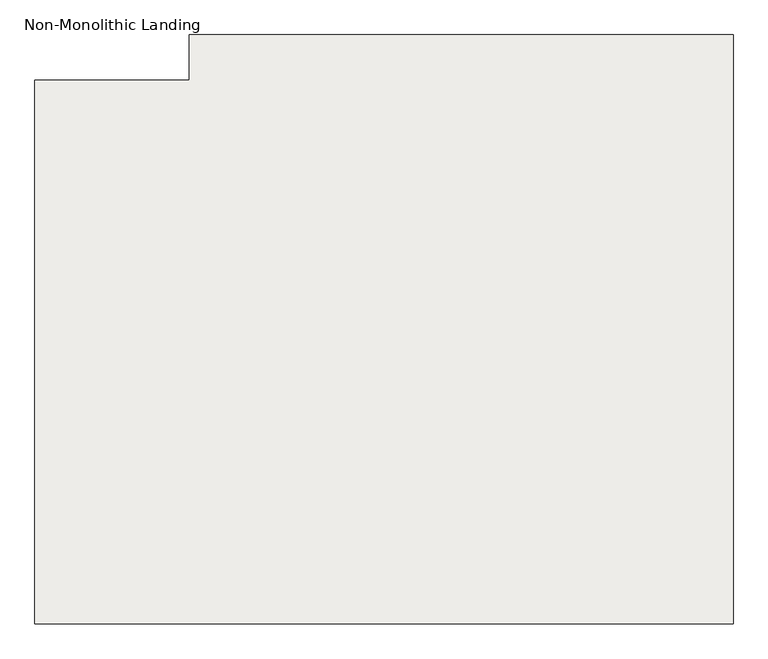
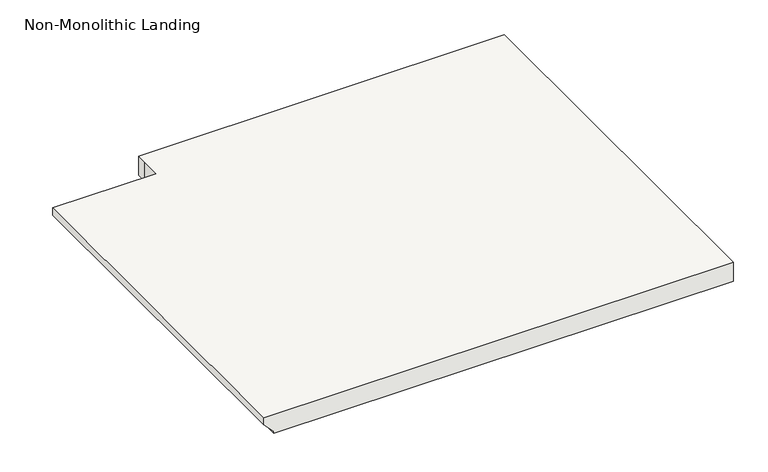
"""IFC4 building model written with IfcOpenShell, lengths in millimetres: slab geometry, Non-Monolithic Landing."""

from ifc_helpers import new_model, si_unit, origin, place, context, project, spatial, faceted_brep, source, transform, mapped, element, save


def non_monolithic_landing_c5e4f846(model_context):
    return source(origin(), model_context, "Body", "Brep", [
        faceted_brep([(9992.8923267, 6928.6147181, 2209.8), (9992.8923267, 7893.8147181, 2209.8), (9992.8923267, 7919.2147181, 2209.8), (9078.4923267, 7919.2147181, 2209.8), (9078.4923267, 7893.8147181, 2209.8), (9078.4923267, 7843.0147181, 2209.8), (8819.4175025, 7843.0147181, 2209.8), (8819.4175025, 6928.6147181, 2209.8), (8844.8175025, 6928.6147181, 2159.0), (8844.8175025, 7843.0147181, 2159.0), (9078.4923267, 7843.0147181, 2159.0), (9078.4923267, 7893.8147181, 2159.0), (9078.4923267, 7919.2147181, 2159.0), (9992.8923267, 7919.2147181, 2159.0), (9992.8923267, 7893.8147181, 2159.0), (9992.8923267, 6928.6147181, 2159.0), (8819.4175025, 6928.6147181, 2190.75), (8844.8175025, 6928.6147181, 2165.35), (8819.4175025, 7843.0147181, 2190.75), (8844.8175025, 7843.0147181, 2165.35)], [[[0, 1, 2, 3, 4, 5, 6, 7]], [[8, 9, 10, 11, 12, 13, 14, 15]], [[0, 7, 16, 17, 8, 15]], [[2, 1, 14, 13]], [[4, 3, 12, 11]], [[5, 4, 11, 10]], [[16, 7, 6, 18]], [[17, 16, 18, 19]], [[9, 8, 17, 19]], [[1, 0, 15, 14]], [[3, 2, 13, 12]], [[6, 5, 10, 9, 19, 18]]]),
    ])


if __name__ == "__main__":
    model = new_model("IFC4")
    model_context = context("Model", 3, world=origin())
    ifc_project = project(units=[si_unit("LENGTHUNIT", "METRE", prefix="MILLI")], contexts=[model_context])
    site = spatial("IfcSite", under=ifc_project)
    building = spatial("IfcBuilding", under=site)
    placement = place(None, origin())
    non_monolithic_landing_shape = non_monolithic_landing_c5e4f846(model_context)
    element("IfcSlab", 1, ObjectType="Non-Monolithic Landing", at=placement, inside=building, context=model_context, shape_type="MappedRepresentation", body=[
        mapped(non_monolithic_landing_shape, transform((0.0, 0.0, 0.0), x_axis=(1.0, 0.0, 0.0), y_axis=(0.0, 1.0, 0.0), z_axis=(0.0, 0.0, 1.0))),
    ])
    save(model, "model.ifc")
